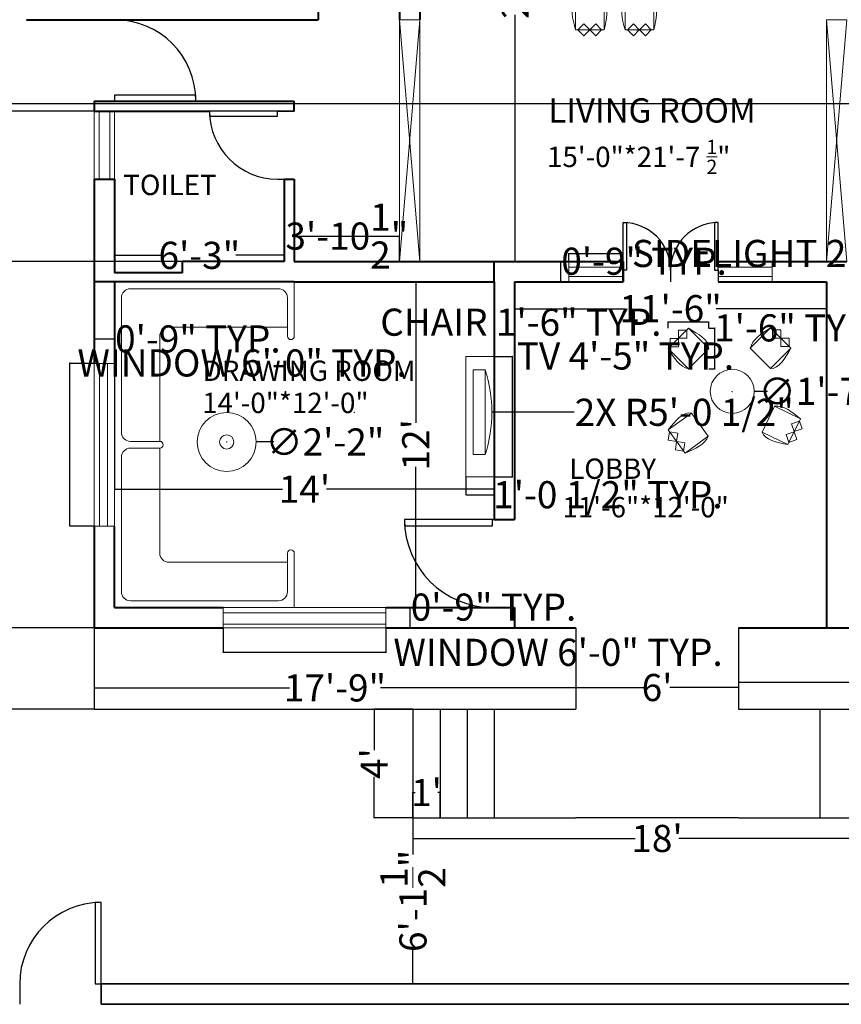
# Model space of a CAD drawing. Units: inches. Extents: x 1146 to 2917, y 889 to 2437.
# Tile 4 of 13: x 1428 to 1792, y 1432 to 1867. Entities that reach past the tile are written whole.
import ezdxf

# ---------------------------------------------------------------- set-up
doc = ezdxf.new("R2010")
doc.units = ezdxf.units.IN
doc.header["$MEASUREMENT"] = 0
for name, color, linetype, lineweight in [('A-ANNO-DIMS', 2, 'Continuous', 18), ('A-ANNO-SYMB', 7, 'Continuous', 25), ('A-AREA-IDEN', 7, 'Continuous', 18), ('A-FURN', 9, 'Continuous', 18), ('A-SITE-GATE', 10, 'Continuous', 25), ('A-SITE-WALL', 7, 'Continuous', 35), ('door', 10, 'Continuous', 25), ('openings', 130, 'Continuous', 18), ('staircase', 6, 'Continuous', 25), ('wall', 7, 'Continuous', 40), ('window', 5, 'Continuous', 18)]:
    doc.layers.add(name, color=color, linetype=linetype, lineweight=lineweight)
doc.styles.get("Standard").update_dxf_attribs({"font": 'arial.ttf'})
doc.dimstyles.get("Standard").update_dxf_attribs({"dimtxt": 12, "dimasz": 0.18, "dimexe": 0.18, "dimexo": 0.0625, "dimgap": 0.09, "dimtad": 0, "dimtoh": 1, "dimdec": 1, "dimzin": 0, "dimdsep": 46, "dimlunit": 4, "dimtxsty": 'Standard', "dimcen": 0.09, "dimadec": 0, "dimazin": 0, "dimtfac": 1, "dimtdec": 1, "dimtofl": 0, "dimtmove": 0, "dimatfit": 3, "dimfxl": 1, "dimtolj": 1, "dimtzin": 0, "dimarcsym": 0})

# ---------------------------------------------------------------- blocks, each defined once
blk = doc.blocks.new('*D9')
at = {"layer": 'A-ANNO-DIMS', "color": 0, "lineweight": -2, "transparency": 16777216}
for p, q in [((1674.13, 1598.33), (1674.13, 1571.83)), ((1746.13, 1598.33), (1746.13, 1571.83)), ((1674.31, 1572.01), (1704.49, 1572.01)), ((1745.95, 1572.01), (1715.78, 1572.01))]:
    blk.add_line(p, q, dxfattribs=at)
at = {"layer": 'A-ANNO-DIMS', "color": 0, "transparency": 16777216}
for points in [[(1674.31, 1572.04), (1674.31, 1571.98), (1674.13, 1572.01)], [(1745.95, 1572.04), (1745.95, 1571.98), (1746.13, 1572.01)]]:
    blk.add_solid(points, dxfattribs=at)
at = {"layer": 'Defpoints', "color": 0, "transparency": 16777216}
for p in [(1674.13, 1598.39), (1746.13, 1598.39), (1746.13, 1572.01)]:
    blk.add_point(p, dxfattribs=at)
at = {"layer": 'A-ANNO-DIMS', "color": 0, "transparency": 16777216, "insert": (1710.13, 1572.01), "char_height": 12, "attachment_point": 5}
blk.add_mtext("\\A1;6'", dxfattribs=at)
blk = doc.blocks.new('*D10')
at = {"layer": 'A-ANNO-DIMS', "color": 0, "lineweight": -2, "transparency": 16777216}
for p, q in [((1461.13, 1598.33), (1461.13, 1571.65)), ((1674.13, 1598.33), (1674.13, 1571.65)), ((1461.31, 1571.83), (1547.5, 1571.83)), ((1673.95, 1571.83), (1587.77, 1571.83))]:
    blk.add_line(p, q, dxfattribs=at)
at = {"layer": 'A-ANNO-DIMS', "color": 0, "transparency": 16777216}
for points in [[(1461.31, 1571.86), (1461.31, 1571.8), (1461.13, 1571.83)], [(1673.95, 1571.86), (1673.95, 1571.8), (1674.13, 1571.83)]]:
    blk.add_solid(points, dxfattribs=at)
at = {"layer": 'Defpoints', "color": 0, "transparency": 16777216}
for p in [(1461.13, 1598.39), (1674.13, 1598.39), (1674.13, 1571.83)]:
    blk.add_point(p, dxfattribs=at)
at = {"layer": 'A-ANNO-DIMS', "color": 0, "transparency": 16777216, "insert": (1567.63, 1571.83), "char_height": 12, "attachment_point": 5}
blk.add_mtext('\\A1;17\'-9"', dxfattribs=at)
blk = doc.blocks.new('*D11')
at = {"layer": 'A-ANNO-DIMS', "color": 0, "lineweight": -2, "transparency": 16777216}
for p, q in [((1746.13, 1598.33), (1746.13, 1574.21)), ((1959.13, 1598.33), (1959.13, 1574.21)), ((1746.31, 1574.39), (1832.5, 1574.39)), ((1958.95, 1574.39), (1872.77, 1574.39))]:
    blk.add_line(p, q, dxfattribs=at)
at = {"layer": 'A-ANNO-DIMS', "color": 0, "transparency": 16777216}
for points in [[(1746.31, 1574.42), (1746.31, 1574.36), (1746.13, 1574.39)], [(1958.95, 1574.42), (1958.95, 1574.36), (1959.13, 1574.39)]]:
    blk.add_solid(points, dxfattribs=at)
at = {"layer": 'Defpoints', "color": 0, "transparency": 16777216}
for p in [(1746.13, 1598.39), (1959.13, 1598.39), (1959.13, 1574.39)]:
    blk.add_point(p, dxfattribs=at)
at = {"layer": 'A-ANNO-DIMS', "color": 0, "transparency": 16777216, "insert": (1852.63, 1574.39), "char_height": 12, "attachment_point": 5}
blk.add_mtext('\\A1;17\'-9"', dxfattribs=at)
blk = doc.blocks.new('*D12')
at = {"layer": 'A-ANNO-DIMS', "color": 0, "lineweight": -2, "transparency": 16777216}
for p, q in [((1602.07, 1562.39), (1584.75, 1562.39)), ((1584.93, 1562.21), (1584.93, 1544.24)), ((1584.93, 1514.57), (1584.93, 1532.54)), ((1602.07, 1514.39), (1584.75, 1514.39))]:
    blk.add_line(p, q, dxfattribs=at)
at = {"layer": 'A-ANNO-DIMS', "color": 0, "transparency": 16777216}
for points in [[(1584.9, 1562.21), (1584.96, 1562.21), (1584.93, 1562.39)], [(1584.9, 1514.57), (1584.96, 1514.57), (1584.93, 1514.39)]]:
    blk.add_solid(points, dxfattribs=at)
at = {"layer": 'Defpoints', "color": 0, "transparency": 16777216}
for p in [(1602.13, 1562.39), (1584.93, 1514.39), (1602.13, 1514.39)]:
    blk.add_point(p, dxfattribs=at)
at = {"layer": 'A-ANNO-DIMS', "color": 0, "transparency": 16777216, "insert": (1584.93, 1538.39), "char_height": 12, "attachment_point": 5, "rotation": 90}
blk.add_mtext("\\A1;4'", dxfattribs=at)
blk = doc.blocks.new('*D13')
at = {"layer": 'A-ANNO-DIMS', "color": 0, "lineweight": -2, "transparency": 16777216}
for p, q in [((1602.13, 1514.45), (1602.13, 1525.77)), ((1602.31, 1525.59), (1603.09, 1525.59)), ((1613.95, 1525.59), (1613.18, 1525.59)), ((1614.13, 1514.45), (1614.13, 1525.77))]:
    blk.add_line(p, q, dxfattribs=at)
at = {"layer": 'A-ANNO-DIMS', "color": 0, "transparency": 16777216}
for points in [[(1602.31, 1525.62), (1602.31, 1525.56), (1602.13, 1525.59)], [(1613.95, 1525.62), (1613.95, 1525.56), (1614.13, 1525.59)]]:
    blk.add_solid(points, dxfattribs=at)
at = {"layer": 'Defpoints', "color": 0, "transparency": 16777216}
for p in [(1614.13, 1525.59), (1602.13, 1514.39), (1614.13, 1514.39)]:
    blk.add_point(p, dxfattribs=at)
at = {"layer": 'A-ANNO-DIMS', "color": 0, "transparency": 16777216, "insert": (1608.13, 1525.59), "char_height": 12, "attachment_point": 5}
blk.add_mtext("\\A1;1'", dxfattribs=at)
blk = doc.blocks.new('*D14')
at = {"layer": 'A-ANNO-DIMS', "color": 0, "lineweight": -2, "transparency": 16777216}
for p, q in [((1602.13, 1514.33), (1602.13, 1505.08)), ((1818.13, 1514.33), (1818.13, 1505.08)), ((1602.31, 1505.26), (1700.43, 1505.26)), ((1817.95, 1505.26), (1719.84, 1505.26))]:
    blk.add_line(p, q, dxfattribs=at)
at = {"layer": 'A-ANNO-DIMS', "color": 0, "transparency": 16777216}
for points in [[(1602.31, 1505.29), (1602.31, 1505.23), (1602.13, 1505.26)], [(1817.95, 1505.29), (1817.95, 1505.23), (1818.13, 1505.26)]]:
    blk.add_solid(points, dxfattribs=at)
at = {"layer": 'Defpoints', "color": 0, "transparency": 16777216}
for p in [(1602.13, 1514.39), (1818.13, 1514.39), (1818.13, 1505.26)]:
    blk.add_point(p, dxfattribs=at)
at = {"layer": 'A-ANNO-DIMS', "color": 0, "transparency": 16777216, "insert": (1710.13, 1505.26), "char_height": 12, "attachment_point": 5}
blk.add_mtext("\\A1;18'", dxfattribs=at)
blk = doc.blocks.new('*D15')
at = {"layer": 'A-ANNO-DIMS', "color": 0, "lineweight": -2, "transparency": 16777216}
for p, q in [((1602.07, 1514.39), (1601.95, 1514.39)), ((1602.13, 1514.21), (1602.13, 1498.09)), ((1602.13, 1441.07), (1602.13, 1457.19)), ((1602.07, 1440.89), (1601.95, 1440.89))]:
    blk.add_line(p, q, dxfattribs=at)
at = {"layer": 'A-ANNO-DIMS', "color": 0, "transparency": 16777216}
for points in [[(1602.1, 1514.21), (1602.16, 1514.21), (1602.13, 1514.39)], [(1602.1, 1441.07), (1602.16, 1441.07), (1602.13, 1440.89)]]:
    blk.add_solid(points, dxfattribs=at)
at = {"layer": 'Defpoints', "color": 0, "transparency": 16777216}
for p in [(1602.13, 1514.39), (1602.13, 1440.89), (1602.13, 1440.89)]:
    blk.add_point(p, dxfattribs=at)
at = {"layer": 'A-ANNO-DIMS', "color": 0, "transparency": 16777216, "insert": (1602.13, 1477.64), "char_height": 12, "attachment_point": 5, "rotation": 90}
blk.add_mtext('\\A1;6\'-1{\\H1x;\\S1/2;}"', dxfattribs=at)
blk = doc.blocks.new('*U22')
for p, q in [((-24, 0), (-24, -6)), ((0, 0), (0, -6))]:
    blk.add_line(p, q)
blk.add_lwpolyline([(0, 0), (0, 24), (-1.75, 24), (-1.75, 0)], close=True)
blk.add_arc((0, 0), 24, 90, 180)
blk = doc.blocks.new('*U18')
for p, q in [((-24, 0), (-24, -6)), ((0, 0), (0, -6))]:
    blk.add_line(p, q)
blk.add_lwpolyline([(0, 0), (0, 24), (-1.75, 24), (-1.75, 0)], close=True)
blk.add_arc((0, 0), 24, 90, 180)
blk = doc.blocks.new('*U21')
for p, q in [((0, 0), (0, 6)), ((24, 0), (24, 6))]:
    blk.add_line(p, q)
blk.add_lwpolyline([(0, 0), (0, -24), (1.75, -24), (1.75, 0)], close=True)
blk.add_arc((0, 0), 24, 270, 0)
blk = doc.blocks.new('*D32')
at = {"layer": 'A-ANNO-DIMS', "color": 0, "lineweight": -2, "transparency": 16777216}
for p, q in [((1470.13, 1760.45), (1470.13, 1763.35)), ((1470.31, 1763.17), (1491.56, 1763.17)), ((1544.95, 1763.17), (1523.71, 1763.17)), ((1545.13, 1760.45), (1545.13, 1763.35))]:
    blk.add_line(p, q, dxfattribs=at)
at = {"layer": 'A-ANNO-DIMS', "color": 0, "transparency": 16777216}
for points in [[(1470.31, 1763.2), (1470.31, 1763.14), (1470.13, 1763.17)], [(1544.95, 1763.2), (1544.95, 1763.14), (1545.13, 1763.17)]]:
    blk.add_solid(points, dxfattribs=at)
at = {"layer": 'Defpoints', "color": 0, "transparency": 16777216}
for p in [(1470.13, 1763.17), (1470.13, 1760.39), (1545.13, 1760.39)]:
    blk.add_point(p, dxfattribs=at)
at = {"layer": 'A-ANNO-DIMS', "color": 0, "transparency": 16777216, "insert": (1507.63, 1763.17), "char_height": 12, "attachment_point": 5}
blk.add_mtext('\\A1;6\'-3"', dxfattribs=at)
blk = doc.blocks.new('*D33')
at = {"layer": 'A-ANNO-DIMS', "color": 0, "lineweight": -2, "transparency": 16777216}
for p, q in [((1549.63, 1760.45), (1549.63, 1771.86)), ((1549.81, 1771.68), (1595.95, 1771.68)), ((1596.13, 1760.45), (1596.13, 1771.86))]:
    blk.add_line(p, q, dxfattribs=at)
at = {"layer": 'A-ANNO-DIMS', "color": 0, "transparency": 16777216}
for points in [[(1549.81, 1771.71), (1549.81, 1771.65), (1549.63, 1771.68)], [(1595.95, 1771.71), (1595.95, 1771.65), (1596.13, 1771.68)]]:
    blk.add_solid(points, dxfattribs=at)
at = {"layer": 'Defpoints', "color": 0, "transparency": 16777216}
for p in [(1596.13, 1771.68), (1549.63, 1760.39), (1596.13, 1760.39)]:
    blk.add_point(p, dxfattribs=at)
at = {"layer": 'A-ANNO-DIMS', "color": 0, "transparency": 16777216, "insert": (1572.88, 1771.68), "char_height": 12, "attachment_point": 5}
blk.add_mtext('\\A1;3\'-10{\\H1x;\\S1/2;}"', dxfattribs=at)
blk = doc.blocks.new('*D39')
at = {"layer": 'A-ANNO-DIMS', "color": 0, "lineweight": -2, "transparency": 16777216}
for p, q in [((1605.2, 2020.39), (1647.47, 2020.39)), ((1647.29, 2020.21), (1647.29, 1911.2)), ((1647.29, 1760.57), (1647.29, 1869.59)), ((1605.2, 1760.39), (1647.47, 1760.39))]:
    blk.add_line(p, q, dxfattribs=at)
at = {"layer": 'A-ANNO-DIMS', "color": 0, "transparency": 16777216}
for points in [[(1647.26, 2020.21), (1647.32, 2020.21), (1647.29, 2020.39)], [(1647.26, 1760.57), (1647.32, 1760.57), (1647.29, 1760.39)]]:
    blk.add_solid(points, dxfattribs=at)
at = {"layer": 'Defpoints', "color": 0, "transparency": 16777216}
for p in [(1605.13, 2020.39), (1605.13, 1760.39), (1647.29, 1760.39)]:
    blk.add_point(p, dxfattribs=at)
at = {"layer": 'A-ANNO-DIMS', "color": 0, "transparency": 16777216, "insert": (1647.29, 1890.39), "char_height": 12, "attachment_point": 5, "rotation": 90}
blk.add_mtext('\\A1;21\'-8"', dxfattribs=at)
blk = doc.blocks.new('*D40')
at = {"layer": 'A-ANNO-DIMS', "color": 0, "lineweight": -2, "transparency": 16777216}
for p, q in [((1470.13, 1751.33), (1470.13, 1659.58)), ((1638.13, 1751.33), (1638.13, 1659.58)), ((1470.31, 1659.76), (1544.43, 1659.76)), ((1637.95, 1659.76), (1563.84, 1659.76))]:
    blk.add_line(p, q, dxfattribs=at)
at = {"layer": 'A-ANNO-DIMS', "color": 0, "transparency": 16777216}
for points in [[(1470.31, 1659.79), (1470.31, 1659.73), (1470.13, 1659.76)], [(1637.95, 1659.79), (1637.95, 1659.73), (1638.13, 1659.76)]]:
    blk.add_solid(points, dxfattribs=at)
at = {"layer": 'Defpoints', "color": 0, "transparency": 16777216}
for p in [(1470.13, 1751.39), (1638.13, 1751.39), (1638.13, 1659.76)]:
    blk.add_point(p, dxfattribs=at)
at = {"layer": 'A-ANNO-DIMS', "color": 0, "transparency": 16777216, "insert": (1554.13, 1659.76), "char_height": 12, "attachment_point": 5}
blk.add_mtext("\\A1;14'", dxfattribs=at)
blk = doc.blocks.new('*D41')
at = {"layer": 'A-ANNO-DIMS', "color": 0, "lineweight": -2, "transparency": 16777216}
for p, q in [((1638.07, 1751.39), (1603.2, 1751.39)), ((1603.38, 1751.21), (1603.38, 1689.1)), ((1603.38, 1607.57), (1603.38, 1669.68)), ((1638.07, 1607.39), (1603.2, 1607.39))]:
    blk.add_line(p, q, dxfattribs=at)
at = {"layer": 'A-ANNO-DIMS', "color": 0, "transparency": 16777216}
for points in [[(1603.35, 1751.21), (1603.41, 1751.21), (1603.38, 1751.39)], [(1603.35, 1607.57), (1603.41, 1607.57), (1603.38, 1607.39)]]:
    blk.add_solid(points, dxfattribs=at)
at = {"layer": 'Defpoints', "color": 0, "transparency": 16777216}
for p in [(1638.13, 1751.39), (1603.38, 1607.39), (1638.13, 1607.39)]:
    blk.add_point(p, dxfattribs=at)
at = {"layer": 'A-ANNO-DIMS', "color": 0, "transparency": 16777216, "insert": (1603.38, 1679.39), "char_height": 12, "attachment_point": 5, "rotation": 90}
blk.add_mtext("\\A1;12'", dxfattribs=at)
blk = doc.blocks.new('*D44')
at = {"layer": 'A-ANNO-DIMS', "color": 0, "lineweight": -2, "transparency": 16777216}
for p, q in [((1647.13, 1751.33), (1647.13, 1739.39)), ((1785.13, 1751.33), (1785.13, 1739.39)), ((1647.31, 1739.57), (1696, 1739.57)), ((1784.95, 1739.57), (1736.27, 1739.57))]:
    blk.add_line(p, q, dxfattribs=at)
at = {"layer": 'A-ANNO-DIMS', "color": 0, "transparency": 16777216}
for points in [[(1647.31, 1739.6), (1647.31, 1739.54), (1647.13, 1739.57)], [(1784.95, 1739.6), (1784.95, 1739.54), (1785.13, 1739.57)]]:
    blk.add_solid(points, dxfattribs=at)
at = {"layer": 'Defpoints', "color": 0, "transparency": 16777216}
for p in [(1647.13, 1751.39), (1785.13, 1751.39), (1785.13, 1739.57)]:
    blk.add_point(p, dxfattribs=at)
at = {"layer": 'A-ANNO-DIMS', "color": 0, "transparency": 16777216, "insert": (1716.13, 1739.57), "char_height": 12, "attachment_point": 5}
blk.add_mtext('\\A1;11\'-6"', dxfattribs=at)
blk = doc.blocks.new('*U17')
for p, q in [((0, 0), (0, -6)), ((24, 0), (24, -6))]:
    blk.add_line(p, q)
blk.add_lwpolyline([(0, 0), (0, 24), (1.75, 24), (1.75, 0)], close=True)
blk.add_arc((0, 0), 24, 0, 90)
blk = doc.blocks.new('CHAIR-LOUNGE')
blk.add_line((0, 8.98), (8.98, 0))
blk.add_lwpolyline([(0, 8.98), (8.98, 17.96), (17.96, 8.98), (8.98, 0)])
for points in [[(9.79, 17.15), (13.47, 17.15), (13.47, 13.47), (9.79, 13.47)], [(13.52, 13.42), (17.2, 13.42), (17.2, 9.74), (13.52, 9.74)]]:
    blk.add_lwpolyline(points, close=True)
for points in [[(8.98, 17.96), (4.93, 15.41), (0.87, 12.85), (0, 8.98)], [(17.96, 8.98), (15.38, 4.49), (12.8, -0.01), (8.98, 0)]]:
    blk.add_open_spline(points, degree=3)
blk = doc.blocks.new('TV-CONSOLE')
for points in [[(0, 53.2), (12.54, 53.2), (12.54, 0), (0, 0)], [(3.13, 47.21), (8.47, 47.21), (8.47, 9.76), (3.13, 9.76)]]:
    blk.add_lwpolyline(points, close=True)
blk.add_arc((-49.25, 28.49), 60.68, 342.0216, 17.9784)
blk = doc.blocks.new('WINDOW-PLAN-72-3')
for points in [[(0, 72), (9, 72), (9, 0), (0, 0)], [(2.34, 72), (5.93, 72), (5.93, 0), (2.34, 0)]]:
    blk.add_lwpolyline(points, close=True)
blk = doc.blocks.new('WINDOW-PLAN-72-4')
for points in [[(0, 9), (72, 9), (72, 0), (0, 0)], [(0, 6.62), (72, 6.62), (72, 1.59), (0, 1.59)]]:
    blk.add_lwpolyline(points, close=True)
blk = doc.blocks.new('SIDELIGHT-PLAN-24')
for points in [[(0, 9), (24, 9), (24, 0), (0, 0)], [(0, 6.5), (24, 6.5), (24, 2.47), (0, 2.47)]]:
    blk.add_lwpolyline(points, close=True)
blk = doc.blocks.new('*D97')
at = {"layer": 'A-ANNO-DIMS', "color": 0, "lineweight": -2, "transparency": 16777216}
for p, q in [((1715.06, 1733.6), (1714.88, 1733.6)), ((1715.06, 1730.96), (1715.06, 1733.78)), ((1732.85, 1733.6), (1715.24, 1733.6)), ((1733.03, 1730.96), (1733.03, 1733.78))]:
    blk.add_line(p, q, dxfattribs=at)
at = {"layer": 'A-ANNO-DIMS', "color": 0, "transparency": 16777216}
for points in [[(1715.24, 1733.63), (1715.24, 1733.57), (1715.06, 1733.6)], [(1732.85, 1733.63), (1732.85, 1733.57), (1733.03, 1733.6)]]:
    blk.add_solid(points, dxfattribs=at)
at = {"layer": 'Defpoints', "color": 0, "transparency": 16777216}
for p in [(1715.06, 1733.6), (1715.06, 1730.9), (1733.03, 1730.9)]:
    blk.add_point(p, dxfattribs=at)
at = {"layer": 'A-ANNO-DIMS', "color": 0, "transparency": 16777216, "insert": (1649.87, 1733.6), "char_height": 12, "attachment_point": 5}
blk.add_mtext('\\A1;CHAIR 1\'-6" TYP.', dxfattribs=at)
blk = doc.blocks.new('*D98')
at = {"layer": 'A-ANNO-DIMS', "color": 0, "lineweight": -2, "transparency": 16777216}
for p, q in [((1733.09, 1730.9), (1735.9, 1730.9)), ((1735.72, 1730.9), (1735.72, 1731.08)), ((1735.72, 1731.08), (1735.9, 1731.08)), ((1735.72, 1713.12), (1735.72, 1730.72)), ((1733.09, 1712.94), (1735.9, 1712.94))]:
    blk.add_line(p, q, dxfattribs=at)
at = {"layer": 'A-ANNO-DIMS', "color": 0, "transparency": 16777216}
for points in [[(1735.69, 1730.72), (1735.75, 1730.72), (1735.72, 1730.9)], [(1735.69, 1713.12), (1735.75, 1713.12), (1735.72, 1712.94)]]:
    blk.add_solid(points, dxfattribs=at)
at = {"layer": 'Defpoints', "color": 0, "transparency": 16777216}
for p in [(1733.03, 1730.9), (1735.72, 1730.9), (1733.03, 1712.94)]:
    blk.add_point(p, dxfattribs=at)
at = {"layer": 'A-ANNO-DIMS', "color": 0, "transparency": 16777216, "insert": (1772, 1731.08), "char_height": 12, "attachment_point": 5}
blk.add_mtext('\\A1;1\'-6" TYP.', dxfattribs=at)
blk = doc.blocks.new('*D107')
at = {"layer": 'A-ANNO-DIMS', "color": 0, "lineweight": -2, "transparency": 16777216}
for p, q in [((1638.2, 1718.46), (1646.29, 1718.46)), ((1646.11, 1718.46), (1646.11, 1718.64)), ((1646.11, 1718.64), (1646.29, 1718.64)), ((1646.11, 1665.44), (1646.11, 1718.28)), ((1638.2, 1665.26), (1646.29, 1665.26))]:
    blk.add_line(p, q, dxfattribs=at)
at = {"layer": 'A-ANNO-DIMS', "color": 0, "transparency": 16777216}
for points in [[(1646.08, 1718.28), (1646.14, 1718.28), (1646.11, 1718.46)], [(1646.08, 1665.44), (1646.14, 1665.44), (1646.11, 1665.26)]]:
    blk.add_solid(points, dxfattribs=at)
at = {"layer": 'Defpoints', "color": 0, "transparency": 16777216}
for p in [(1638.13, 1718.46), (1646.11, 1718.46), (1638.13, 1665.26)]:
    blk.add_point(p, dxfattribs=at)
at = {"layer": 'A-ANNO-DIMS', "color": 0, "transparency": 16777216, "insert": (1696.15, 1718.64), "char_height": 12, "attachment_point": 5}
blk.add_mtext('\\A1;TV 4\'-5" TYP.', dxfattribs=at)
blk = doc.blocks.new('*D108')
at = {"layer": 'A-ANNO-DIMS', "color": 0, "lineweight": -2, "transparency": 16777216}
for p, q in [((1625.59, 1665.19), (1625.59, 1657.1)), ((1638.13, 1665.19), (1638.13, 1657.1)), ((1625.77, 1657.28), (1637.95, 1657.28)), ((1638.13, 1657.28), (1638.31, 1657.28))]:
    blk.add_line(p, q, dxfattribs=at)
at = {"layer": 'A-ANNO-DIMS', "color": 0, "transparency": 16777216}
for points in [[(1625.77, 1657.31), (1625.77, 1657.25), (1625.59, 1657.28)], [(1637.95, 1657.31), (1637.95, 1657.25), (1638.13, 1657.28)]]:
    blk.add_solid(points, dxfattribs=at)
at = {"layer": 'Defpoints', "color": 0, "transparency": 16777216}
for p in [(1625.59, 1665.26), (1638.13, 1665.26), (1638.13, 1657.28)]:
    blk.add_point(p, dxfattribs=at)
at = {"layer": 'A-ANNO-DIMS', "color": 0, "transparency": 16777216, "insert": (1688.39, 1657.28), "char_height": 12, "attachment_point": 5}
blk.add_mtext('\\A1;1\'-0 1/2" TYP.', dxfattribs=at)
blk = doc.blocks.new('*D113')
at = {"layer": 'A-ANNO-DIMS', "color": 0, "lineweight": -2, "transparency": 16777216}
for p, q in [((1461.07, 1715.39), (1450.15, 1715.39)), ((1450.33, 1715.39), (1450.33, 1715.57)), ((1450.33, 1715.57), (1450.51, 1715.57)), ((1450.33, 1643.57), (1450.33, 1715.21)), ((1461.07, 1643.39), (1450.15, 1643.39))]:
    blk.add_line(p, q, dxfattribs=at)
at = {"layer": 'A-ANNO-DIMS', "color": 0, "transparency": 16777216}
for points in [[(1450.3, 1715.21), (1450.36, 1715.21), (1450.33, 1715.39)], [(1450.3, 1643.57), (1450.36, 1643.57), (1450.33, 1643.39)]]:
    blk.add_solid(points, dxfattribs=at)
at = {"layer": 'Defpoints', "color": 0, "transparency": 16777216}
for p in [(1450.33, 1715.39), (1461.13, 1715.39), (1461.13, 1643.39)]:
    blk.add_point(p, dxfattribs=at)
at = {"layer": 'A-ANNO-DIMS', "color": 0, "transparency": 16777216, "insert": (1526.53, 1715.57), "char_height": 12, "attachment_point": 5}
blk.add_mtext('\\A1;WINDOW 6\'-0" TYP.', dxfattribs=at)
blk = doc.blocks.new('*D114')
at = {"layer": 'A-ANNO-DIMS', "color": 0, "lineweight": -2, "transparency": 16777216}
for p, q in [((1461.13, 1715.45), (1461.13, 1726.37)), ((1461.31, 1726.19), (1469.95, 1726.19)), ((1470.13, 1715.45), (1470.13, 1726.37)), ((1470.13, 1726.19), (1470.31, 1726.19))]:
    blk.add_line(p, q, dxfattribs=at)
at = {"layer": 'A-ANNO-DIMS', "color": 0, "transparency": 16777216}
for points in [[(1461.31, 1726.22), (1461.31, 1726.16), (1461.13, 1726.19)], [(1469.95, 1726.22), (1469.95, 1726.16), (1470.13, 1726.19)]]:
    blk.add_solid(points, dxfattribs=at)
at = {"layer": 'Defpoints', "color": 0, "transparency": 16777216}
for p in [(1470.13, 1726.19), (1461.13, 1715.39), (1470.13, 1715.39)]:
    blk.add_point(p, dxfattribs=at)
at = {"layer": 'A-ANNO-DIMS', "color": 0, "transparency": 16777216, "insert": (1506.98, 1726.19), "char_height": 12, "attachment_point": 5}
blk.add_mtext('\\A1;0\'-9" TYP.', dxfattribs=at)
blk = doc.blocks.new('*D115')
at = {"layer": 'A-ANNO-DIMS', "color": 0, "lineweight": -2, "transparency": 16777216}
for p, q in [((1518.13, 1598.33), (1518.13, 1587.41)), ((1590.13, 1598.33), (1590.13, 1587.41)), ((1518.31, 1587.59), (1589.95, 1587.59)), ((1590.13, 1587.59), (1590.31, 1587.59))]:
    blk.add_line(p, q, dxfattribs=at)
at = {"layer": 'A-ANNO-DIMS', "color": 0, "transparency": 16777216}
for points in [[(1518.31, 1587.62), (1518.31, 1587.56), (1518.13, 1587.59)], [(1589.95, 1587.62), (1589.95, 1587.56), (1590.13, 1587.59)]]:
    blk.add_solid(points, dxfattribs=at)
at = {"layer": 'Defpoints', "color": 0, "transparency": 16777216}
for p in [(1518.13, 1598.39), (1590.13, 1598.39), (1590.13, 1587.59)]:
    blk.add_point(p, dxfattribs=at)
at = {"layer": 'A-ANNO-DIMS', "color": 0, "transparency": 16777216, "insert": (1666.33, 1587.59), "char_height": 12, "attachment_point": 5}
blk.add_mtext('\\A1;WINDOW 6\'-0" TYP.', dxfattribs=at)
blk = doc.blocks.new('*D116')
at = {"layer": 'A-ANNO-DIMS', "color": 0, "lineweight": -2, "transparency": 16777216}
for p, q in [((1590.2, 1607.39), (1601.11, 1607.39)), ((1600.93, 1607.39), (1600.93, 1607.57)), ((1600.93, 1607.57), (1601.11, 1607.57)), ((1600.93, 1598.57), (1600.93, 1607.21)), ((1590.2, 1598.39), (1601.11, 1598.39))]:
    blk.add_line(p, q, dxfattribs=at)
at = {"layer": 'A-ANNO-DIMS', "color": 0, "transparency": 16777216}
for points in [[(1600.9, 1607.21), (1600.96, 1607.21), (1600.93, 1607.39)], [(1600.9, 1598.57), (1600.96, 1598.57), (1600.93, 1598.39)]]:
    blk.add_solid(points, dxfattribs=at)
at = {"layer": 'Defpoints', "color": 0, "transparency": 16777216}
for p in [(1590.13, 1607.39), (1600.93, 1607.39), (1590.13, 1598.39)]:
    blk.add_point(p, dxfattribs=at)
at = {"layer": 'A-ANNO-DIMS', "color": 0, "transparency": 16777216, "insert": (1637.78, 1607.57), "char_height": 12, "attachment_point": 5}
blk.add_mtext('\\A1;0\'-9" TYP.', dxfattribs=at)
blk = doc.blocks.new('*D117')
at = {"layer": 'A-ANNO-DIMS', "color": 0, "lineweight": -2, "transparency": 16777216}
for p, q in [((1671.13, 1760.45), (1671.13, 1764.17)), ((1671.31, 1763.99), (1694.95, 1763.99)), ((1695.13, 1760.45), (1695.13, 1764.17)), ((1695.13, 1763.99), (1695.31, 1763.99))]:
    blk.add_line(p, q, dxfattribs=at)
at = {"layer": 'A-ANNO-DIMS', "color": 0, "transparency": 16777216}
for points in [[(1671.31, 1764.02), (1671.31, 1763.96), (1671.13, 1763.99)], [(1694.95, 1764.02), (1694.95, 1763.96), (1695.13, 1763.99)]]:
    blk.add_solid(points, dxfattribs=at)
at = {"layer": 'Defpoints', "color": 0, "transparency": 16777216}
for p in [(1695.13, 1763.99), (1671.13, 1760.39), (1695.13, 1760.39)]:
    blk.add_point(p, dxfattribs=at)
at = {"layer": 'A-ANNO-DIMS', "color": 0, "transparency": 16777216, "insert": (1778.52, 1763.99), "char_height": 12, "attachment_point": 5}
blk.add_mtext('\\A1;SIDELIGHT 2\'-0" TYP.', dxfattribs=at)
blk = doc.blocks.new('*D118')
at = {"layer": 'A-ANNO-DIMS', "color": 0, "lineweight": -2, "transparency": 16777216}
for p, q in [((1671.07, 1760.39), (1667.35, 1760.39)), ((1667.53, 1760.39), (1667.53, 1760.57)), ((1667.53, 1760.57), (1667.71, 1760.57)), ((1667.53, 1751.57), (1667.53, 1760.21)), ((1671.07, 1751.39), (1667.35, 1751.39))]:
    blk.add_line(p, q, dxfattribs=at)
at = {"layer": 'A-ANNO-DIMS', "color": 0, "transparency": 16777216}
for points in [[(1667.5, 1760.21), (1667.56, 1760.21), (1667.53, 1760.39)], [(1667.5, 1751.57), (1667.56, 1751.57), (1667.53, 1751.39)]]:
    blk.add_solid(points, dxfattribs=at)
at = {"layer": 'Defpoints', "color": 0, "transparency": 16777216}
for p in [(1667.53, 1760.39), (1671.13, 1760.39), (1671.13, 1751.39)]:
    blk.add_point(p, dxfattribs=at)
at = {"layer": 'A-ANNO-DIMS', "color": 0, "transparency": 16777216, "insert": (1704.38, 1760.57), "char_height": 12, "attachment_point": 5}
blk.add_mtext('\\A1;0\'-9" TYP.', dxfattribs=at)
blk = doc.blocks.new('*D170')
at = {"layer": 'A-ANNO-DIMS', "color": 0, "lineweight": -2, "transparency": 16777216}
for p, q in [((1461.07, 1598.39), (1163.51, 1598.39)), ((1163.69, 1598.21), (1163.69, 1596.43)), ((1163.69, 1562.57), (1163.69, 1564.36)), ((1461.07, 1562.39), (1163.51, 1562.39))]:
    blk.add_line(p, q, dxfattribs=at)
at = {"layer": 'A-ANNO-DIMS', "color": 0, "transparency": 16777216}
for points in [[(1163.66, 1598.21), (1163.72, 1598.21), (1163.69, 1598.39)], [(1163.66, 1562.57), (1163.72, 1562.57), (1163.69, 1562.39)]]:
    blk.add_solid(points, dxfattribs=at)
at = {"layer": 'Defpoints', "color": 0, "transparency": 16777216}
for p in [(1461.13, 1598.39), (1163.69, 1562.39), (1461.13, 1562.39)]:
    blk.add_point(p, dxfattribs=at)
at = {"layer": 'A-ANNO-DIMS', "color": 0, "transparency": 16777216, "insert": (1163.69, 1580.39), "char_height": 12, "attachment_point": 5, "rotation": 90}
blk.add_mtext('\\A1;3\'-0"', dxfattribs=at)
blk = doc.blocks.new('*D171')
at = {"layer": 'A-ANNO-DIMS', "color": 0, "lineweight": -2, "transparency": 16777216}
for p, q in [((1549.57, 1826.89), (1163.51, 1826.89)), ((1163.69, 1826.71), (1163.69, 1823.66)), ((1545.07, 1760.39), (1163.51, 1760.39)), ((1163.69, 1760.57), (1163.69, 1763.62))]:
    blk.add_line(p, q, dxfattribs=at)
at = {"layer": 'A-ANNO-DIMS', "color": 0, "transparency": 16777216}
for points in [[(1163.66, 1826.71), (1163.72, 1826.71), (1163.69, 1826.89)], [(1163.66, 1760.57), (1163.72, 1760.57), (1163.69, 1760.39)]]:
    blk.add_solid(points, dxfattribs=at)
at = {"layer": 'Defpoints', "color": 0, "transparency": 16777216}
for p in [(1549.63, 1826.89), (1163.69, 1760.39), (1545.13, 1760.39)]:
    blk.add_point(p, dxfattribs=at)
at = {"layer": 'A-ANNO-DIMS', "color": 0, "transparency": 16777216, "insert": (1163.69, 1793.64), "char_height": 12, "attachment_point": 5, "rotation": 90}
blk.add_mtext('\\A1;5\'-6 1/2"', dxfattribs=at)
blk = doc.blocks.new('*D176')
at = {"layer": 'A-ANNO-DIMS', "color": 0, "lineweight": -2, "transparency": 16777216}
for p, q in [((1576.25, 1693.74), (1576.43, 1693.74)), ((1576.34, 1693.65), (1576.34, 1693.83)), ((1673.42, 1693.74), (1637.2, 1693.74))]:
    blk.add_line(p, q, dxfattribs=at)
at = {"layer": 'A-ANNO-DIMS', "color": 0, "transparency": 16777216}
blk.add_solid([(1637.2, 1693.77), (1637.2, 1693.71), (1637.02, 1693.74)], dxfattribs=at)
at = {"layer": 'Defpoints', "color": 0, "transparency": 16777216}
for p in [(1576.34, 1693.74), (1637.02, 1693.74)]:
    blk.add_point(p, dxfattribs=at)
at = {"layer": 'A-ANNO-DIMS', "color": 0, "transparency": 16777216, "insert": (1722.18, 1693.74), "char_height": 12, "attachment_point": 5}
blk.add_mtext('\\A1;2X R5\'-0 1/2"', dxfattribs=at)
blk = doc.blocks.new('*D179')
at = {"layer": 'A-ANNO-DIMS', "color": 0, "lineweight": -2, "transparency": 16777216}
for p, q in [((1519.64, 1680.61), (1519.82, 1680.61)), ((1519.73, 1680.52), (1519.73, 1680.7)), ((1540.64, 1680.61), (1532.98, 1680.61))]:
    blk.add_line(p, q, dxfattribs=at)
at = {"layer": 'A-ANNO-DIMS', "color": 0, "transparency": 16777216}
blk.add_solid([(1532.98, 1680.64), (1532.98, 1680.58), (1532.8, 1680.61)], dxfattribs=at)
at = {"layer": 'Defpoints', "color": 0, "transparency": 16777216}
for p in [(1506.66, 1680.61), (1532.8, 1680.61)]:
    blk.add_point(p, dxfattribs=at)
at = {"layer": 'A-ANNO-DIMS', "color": 0, "transparency": 16777216, "insert": (1563.2, 1680.61), "char_height": 12, "attachment_point": 5}
blk.add_mtext('\\A1;∅2\'-2"', dxfattribs=at)
blk = doc.blocks.new('*D181')
at = {"layer": 'A-ANNO-DIMS', "color": 0, "lineweight": -2, "transparency": 16777216}
for p, q in [((1743.32, 1703), (1743.5, 1703)), ((1743.41, 1702.91), (1743.41, 1703.09)), ((1758.97, 1703), (1753.31, 1703))]:
    blk.add_line(p, q, dxfattribs=at)
at = {"layer": 'A-ANNO-DIMS', "color": 0, "transparency": 16777216}
blk.add_solid([(1753.31, 1703.03), (1753.31, 1702.97), (1753.13, 1703)], dxfattribs=at)
at = {"layer": 'Defpoints', "color": 0, "transparency": 16777216}
for p in [(1733.68, 1703), (1753.13, 1703)]:
    blk.add_point(p, dxfattribs=at)
at = {"layer": 'A-ANNO-DIMS', "color": 0, "transparency": 16777216, "insert": (1795.52, 1703), "char_height": 12, "attachment_point": 5}
blk.add_mtext('\\A1;∅1\'-7 1/2"', dxfattribs=at)

msp = doc.modelspace()

# ---------------------------------------------------------------- linework, layer by layer
at = {"layer": 'A-ANNO-SYMB'}
msp.add_line((1232.84, 1830.35), (2074.15, 1830.35), dxfattribs=at)
at = {"layer": 'A-FURN'}
for p, q in [((1549.63, 1751.39), (1549.63, 1727.39)), ((1542.63, 1748.39), (1477.13, 1748.39)), ((1473.13, 1744.39), (1473.13, 1684.89)), ((1546.63, 1744.39), (1546.63, 1727.39)), ((1546.63, 1731.39), (1494.13, 1731.39)), ((1490.13, 1727.39), (1490.13, 1680.89)), ((1477.13, 1680.89), (1490.13, 1680.89)), ((1477.13, 1677.89), (1490.13, 1677.89)), ((1490.13, 1677.89), (1490.13, 1631.39)), ((1473.13, 1673.89), (1473.13, 1614.39)), ((1546.63, 1614.39), (1546.63, 1631.39)), ((1549.63, 1607.39), (1549.63, 1631.39)), ((1494.13, 1627.39), (1546.63, 1627.39)), ((1477.13, 1610.39), (1542.63, 1610.39))]:
    msp.add_line(p, q, dxfattribs=at)
for centre, radius in [((1743.41, 1703), 9.73), ((1519.73, 1680.61), 13.07), ((1519.73, 1680.61), 3.13)]:
    msp.add_circle(centre, radius, dxfattribs=at)
for centre, radius, start, end in [((1477.13, 1744.39), 4, 90, 180), ((1542.63, 1744.39), 4, 0, 90), ((1494.13, 1727.39), 4, 90, 180), ((1548.13, 1727.39), 1.5, 180, 0), ((1477.13, 1684.89), 4, 180, 270), ((1477.13, 1673.89), 4, 90, 180), ((1490.13, 1679.39), 1.5, 270, 90), ((1494.13, 1631.39), 4, 180, 270), ((1548.13, 1631.39), 1.5, 0, 180), ((1477.13, 1614.39), 4, 180, 270), ((1542.63, 1614.39), 4, 270, 0)]:
    msp.add_arc(centre, radius, start, end, dxfattribs=at)
at = {"layer": 'A-SITE-WALL'}
for p, q in [((1464.13, 1440.89), (1464.13, 1431.89)), ((1464.13, 1440.89), (1896.13, 1440.89)), ((1464.13, 1431.89), (1896.13, 1431.89))]:
    msp.add_line(p, q, dxfattribs=at)
at = {"layer": 'openings'}
for p, q in [((1596.13, 1867.39), (1596.13, 1760.39)), ((1596.13, 1867.39), (1605.13, 1760.39)), ((1596.13, 1760.39), (1605.13, 1867.39)), ((1605.13, 1867.39), (1596.13, 1867.39)), ((1605.13, 1760.39), (1605.13, 1867.39)), ((1785.13, 1867.39), (1785.13, 1760.39)), ((1785.13, 1867.39), (1794.13, 1760.39)), ((1785.13, 1760.39), (1794.13, 1867.39)), ((1785.13, 1867.39), (1794.13, 1867.39)), ((1605.13, 1760.39), (1596.13, 1760.39)), ((1794.13, 1760.39), (1785.13, 1760.39))]:
    msp.add_line(p, q, dxfattribs=at)
at = {"layer": 'staircase'}
for p, q in [((1461.13, 1598.39), (1461.13, 1562.39)), ((1674.13, 1598.39), (1674.13, 1562.39)), ((1746.13, 1598.39), (1746.13, 1562.39)), ((1461.13, 1562.39), (1674.13, 1562.39)), ((1602.13, 1562.39), (1602.13, 1514.39)), ((1614.13, 1562.39), (1614.13, 1514.39)), ((1626.13, 1562.39), (1626.13, 1514.39)), ((1638.13, 1562.39), (1638.13, 1514.39)), ((1746.13, 1562.39), (1959.13, 1562.39)), ((1782.13, 1562.39), (1782.13, 1514.39)), ((1602.13, 1514.39), (1674.13, 1514.39)), ((1746.13, 1514.39), (1674.13, 1514.39)), ((1746.13, 1514.39), (1818.13, 1514.39))]:
    msp.add_line(p, q, dxfattribs=at)
at = {"layer": 'wall'}
for p, q in [((1596.13, 2020.39), (1596.13, 1867.39)), ((1605.13, 2020.39), (1605.13, 1867.39)), ((1560.13, 1876.39), (1560.13, 1867.39)), ((1431.13, 1867.39), (1560.13, 1867.39)), ((1461.13, 1831.39), (1461.13, 1826.89)), ((1461.13, 1831.39), (1549.63, 1831.39)), ((1549.63, 1826.89), (1549.63, 1831.39)), ((1461.13, 1826.89), (1512.13, 1826.89)), ((1461.13, 1796.89), (1470.13, 1796.89)), ((1461.13, 1796.89), (1461.13, 1715.39)), ((1470.13, 1796.89), (1470.13, 1755.39)), ((1545.13, 1796.89), (1545.13, 1760.39)), ((1545.13, 1796.89), (1549.63, 1796.89)), ((1549.63, 1796.89), (1549.63, 1760.39)), ((1545.13, 1760.39), (1500.12, 1760.39)), ((1500.12, 1755.39), (1500.12, 1760.39)), ((1549.63, 1760.39), (1695.13, 1760.39)), ((1638.13, 1751.39), (1638.13, 1760.39)), ((1695.13, 1751.39), (1695.13, 1760.39)), ((1695.13, 1760.39), (1695.13, 1751.39)), ((1737.13, 1760.39), (1794.13, 1760.39)), ((1500.12, 1755.39), (1470.13, 1755.39)), ((1470.13, 1751.39), (1461.13, 1751.39)), ((1549.63, 1751.39), (1470.13, 1751.39)), ((1470.13, 1751.39), (1470.13, 1715.39)), ((1549.63, 1751.39), (1638.13, 1751.39)), ((1638.13, 1751.39), (1638.13, 1646.39)), ((1647.13, 1751.39), (1647.13, 1646.39)), ((1647.13, 1751.39), (1695.13, 1751.39)), ((1737.13, 1751.39), (1785.13, 1751.39)), ((1785.13, 1751.39), (1785.13, 1598.39)), ((1638.13, 1646.39), (1647.13, 1646.39)), ((1461.13, 1643.39), (1461.13, 1598.39)), ((1470.13, 1607.39), (1470.13, 1643.39)), ((1470.13, 1607.39), (1518.13, 1607.39)), ((1590.13, 1607.39), (1647.13, 1607.39)), ((1647.13, 1607.39), (1647.13, 1598.39)), ((1461.13, 1598.39), (1518.13, 1598.39)), ((1590.13, 1598.39), (1674.13, 1598.39)), ((1746.13, 1598.39), (1785.13, 1598.39)), ((1785.13, 1598.39), (1836.13, 1598.39))]:
    msp.add_line(p, q, dxfattribs=at)
at = {"layer": 'window'}
for points in [[(1461.13, 1826.89), (1470.13, 1826.89), (1470.13, 1796.89), (1461.13, 1796.89)], [(1463.36, 1826.89), (1468.02, 1826.89), (1468.02, 1796.89), (1463.36, 1796.89)]]:
    msp.add_lwpolyline(points, close=True, dxfattribs=at)

# ---------------------------------------------------------------- block references
at = {"layer": 'A-FURN'}
for p, rotation in [((1680.42, 1881.94), 224.999999999996), ((1702.35, 1881.94), 224.999999999997), ((1733.02, 1712.94), 89.99999999999856), ((1753.68, 1693.51), 289.1017886992096), ((1734.18, 1692.03), 171.1152140140269)]:
    msp.add_blockref('CHAIR-LOUNGE', p, dxfattribs=dict(at, rotation=rotation))
for name, p in [('CHAIR-LOUNGE', (1751.38, 1713.13)), ('TV-CONSOLE', (1625.59, 1665.26))]:
    msp.add_blockref(name, p, dxfattribs=at)
at = {"layer": 'A-SITE-GATE', "xscale": 1.500000000000009, "yscale": 1.500000000000009, "zscale": 1.500000000000009}
msp.add_blockref('*U18', (1464.13, 1440.89), dxfattribs=at)
at = {"layer": 'door'}
for name, p, xscale, yscale, zscale in [('*U18', (1596.13, 1876.39), 1.500000000000009, 1.500000000000009, 1.500000000000009), ('*U17', (1695.13, 1756.64), 0.8749999999999905, 0.8749999999999905, 0.8749999999999905), ('*U18', (1737.13, 1756.64), 0.8749999999999905, 0.8749999999999905, 0.8749999999999905)]:
    msp.add_blockref(name, p, dxfattribs=dict(at, xscale=xscale, yscale=yscale, zscale=zscale))
at = {"layer": 'door', "rotation": 90}
for name, p, xscale, yscale, zscale in [('*U21', (1470.13, 1831.39), 1.500000000000009, 1.500000000000009, 1.500000000000009), ('*U22', (1542.13, 1826.89), 1.250039435765822, 1.250039435765822, 1.250039435765822), ('*U22', (1637.38, 1646.39), 1.624999999999989, 1.624999999999989, 1.624999999999989)]:
    msp.add_blockref(name, p, dxfattribs=dict(at, xscale=xscale, yscale=yscale, zscale=zscale))
at = {"layer": 'window'}
for name, p in [('SIDELIGHT-PLAN-24', (1671.13, 1751.39)), ('SIDELIGHT-PLAN-24', (1737.13, 1751.39)), ('WINDOW-PLAN-72-3', (1461.13, 1643.39)), ('WINDOW-PLAN-72-4', (1518.13, 1598.39))]:
    msp.add_blockref(name, p, dxfattribs=at)

# ---------------------------------------------------------------- texts
at = {"layer": 'A-AREA-IDEN', "attachment_point": 1}
for s, width, gutter_width, insert, char_height in [('LIVING ROOM', 5487.0895, 53.67, (1661.99, 1832.61), 10.7339), ('\\A1;{\\H45x;15\'-0"*21\'-7 \\H0.7x;\\S1/2;\\H1.42857x;"}', 101.9579, 1, (1661.46, 1814.28), 0.2), ('TOILET', 41.0813, 1, (1473.97, 1798.82), 9), ('DRAWING ROOM', 107.8265, 1, (1509.09, 1716.62), 9), ('14\'-0"*12\'-0"', 84.3913, 1, (1508.89, 1702.39), 9), ('LOBBY', 108.5726, 1, (1671.28, 1673.3), 9), ('11\'-6"*12\'-0"', 89.8445, 1, (1668.28, 1656.29), 9)]:
    msp.add_mtext_dynamic_manual_height_columns(s, width=width, gutter_width=gutter_width, heights=[0], dxfattribs=dict(at, insert=insert, char_height=char_height))

# ---------------------------------------------------------------- dimensions: what is measured, and where the dimension line sits
at = {"layer": 'A-ANNO-DIMS'}
for p1, p2, distance, picture, middle in [((1605.13, 2020.39), (1605.13, 1760.39), 42.15, '*D39', (1647.29, 1890.39)), ((1638.13, 1751.39), (1638.13, 1607.39), -34.75, '*D41', (1603.38, 1679.39)), ((1647.13, 1751.39), (1785.13, 1751.39), -11.82, '*D44', (1716.13, 1739.57)), ((1461.13, 1598.39), (1674.13, 1598.39), -26.56, '*D10', (1567.63, 1571.83)), ((1674.13, 1598.39), (1746.13, 1598.39), -26.38, '*D9', (1710.13, 1572.01)), ((1746.13, 1598.39), (1959.13, 1598.39), -24, '*D11', (1852.63, 1574.39)), ((1602.13, 1562.39), (1602.13, 1514.39), -17.2, '*D12', (1584.93, 1538.39)), ((1602.13, 1514.39), (1614.13, 1514.39), 11.2, '*D13', (1608.13, 1525.59)), ((1602.13, 1514.39), (1818.13, 1514.39), -9.13, '*D14', (1710.13, 1505.26))]:
    dim = msp.add_aligned_dim(p1=p1, p2=p2, distance=distance, dimstyle='Standard', override={"dimclrd": 0, "dimclre": 0, "dimclrt": 0}, dxfattribs=at)
    dim.commit()
    dim.dimension.update_dxf_attribs({"geometry": picture, "text_midpoint": middle})
for base, p1, p2, picture, middle in [((1163.69, 1760.39), (1549.63, 1826.89), (1545.13, 1760.39), '*D171', (1163.69, 1793.64)), ((1163.69, 1562.39), (1461.13, 1598.39), (1461.13, 1562.39), '*D170', (1163.69, 1580.39))]:
    dim = msp.add_linear_dim(base=base, p1=p1, p2=p2, angle=90, dimstyle='Standard', override={"dimdec": 1, "dimlfac": 1, "dimrnd": 0, "dimzin": 1, "dimdsep": 46, "dimlunit": 4, "dimfrac": 2}, dxfattribs=at)
    dim.commit()
    dim.dimension.update_dxf_attribs({"geometry": picture, "text_midpoint": middle})
for base, p1, p2, text, picture, middle in [((1695.13, 1763.99), (1671.13, 1760.39), (1695.13, 1760.39), 'SIDELIGHT <> TYP.', '*D117', (1778.52, 1763.99)), ((1470.13, 1726.19), (1461.13, 1715.39), (1470.13, 1715.39), '<> TYP.', '*D114', (1506.98, 1726.19)), ((1638.13, 1657.28), (1625.59, 1665.26), (1638.13, 1665.26), '<> TYP.', '*D108', (1688.39, 1657.28)), ((1590.13, 1587.59), (1518.13, 1598.39), (1590.13, 1598.39), 'WINDOW <> TYP.', '*D115', (1666.33, 1587.59))]:
    dim = msp.add_linear_dim(base=base, p1=p1, p2=p2, text=text, dimstyle='Standard', override={"dimdec": 1, "dimlfac": 1, "dimrnd": 0, "dimzin": 1, "dimdsep": 46, "dimlunit": 4, "dimfrac": 2}, dxfattribs=at)
    dim.commit()
    dim.dimension.update_dxf_attribs({"geometry": picture, "text_midpoint": middle})
for base, p1, p2, angle, picture, middle in [((1596.13, 1771.68), (1549.63, 1760.39), (1596.13, 1760.39), 0, '*D33', (1572.88, 1771.68)), ((1470.13, 1763.17), (1545.13, 1760.39), (1470.13, 1760.39), 180, '*D32', (1507.63, 1763.17)), ((1638.13, 1659.76), (1470.13, 1751.39), (1638.13, 1751.39), 0, '*D40', (1554.13, 1659.76)), ((1602.13, 1440.89), (1602.13, 1514.39), (1602.13, 1440.89), 270, '*D15', (1602.13, 1477.64))]:
    dim = msp.add_linear_dim(base=base, p1=p1, p2=p2, angle=angle, dimstyle='Standard', override={"dimclrd": 0, "dimclre": 0, "dimclrt": 0}, dxfattribs=at)
    dim.commit()
    dim.dimension.update_dxf_attribs({"geometry": picture, "text_midpoint": middle, "dimtype": 161})
for base, p1, p2, angle, text, picture, middle in [((1667.53, 1760.39), (1671.13, 1751.39), (1671.13, 1760.39), 90, '<> TYP.', '*D118', (1704.38, 1760.57)), ((1715.06, 1733.6), (1733.03, 1730.9), (1715.06, 1730.9), 180, 'CHAIR <> TYP.', '*D97', (1649.87, 1733.6)), ((1646.11, 1718.46), (1638.13, 1665.26), (1638.13, 1718.46), 90, 'TV <> TYP.', '*D107', (1696.15, 1718.64)), ((1735.72, 1730.9), (1733.03, 1712.94), (1733.03, 1730.9), 90, '<> TYP.', '*D98', (1772, 1731.08)), ((1450.33, 1715.39), (1461.13, 1643.39), (1461.13, 1715.39), 90, 'WINDOW <> TYP.', '*D113', (1526.53, 1715.57)), ((1600.93, 1607.39), (1590.13, 1598.39), (1590.13, 1607.39), 90, '<> TYP.', '*D116', (1637.78, 1607.57))]:
    dim = msp.add_linear_dim(base=base, p1=p1, p2=p2, angle=angle, text=text, dimstyle='Standard', override={"dimdec": 1, "dimlfac": 1, "dimrnd": 0, "dimzin": 1, "dimdsep": 46, "dimlunit": 4, "dimfrac": 2}, dxfattribs=at)
    dim.commit()
    dim.dimension.update_dxf_attribs({"geometry": picture, "text_midpoint": middle})
dim = msp.add_radius_dim(center=(1576.34, 1693.74), mpoint=(1637.02, 1693.74), text='2X <>', dimstyle='Standard', override={"dimdec": 1, "dimlfac": 1, "dimrnd": 0, "dimzin": 1, "dimdsep": 46, "dimlunit": 4, "dimfrac": 2}, dxfattribs=at)
dim.commit()
dim.dimension.update_dxf_attribs({"geometry": '*D176', "text_midpoint": (1673.42, 1693.74), "dimtype": 164})
for p1, p2, picture, middle in [((1733.6758, 1702.9975), (1753.135, 1702.998), '*D181', (1758.9728, 1702.9981)), ((1506.66, 1680.61), (1532.8, 1680.61), '*D179', (1540.64, 1680.61))]:
    dim = msp.add_diameter_dim_2p(p1=p1, p2=p2, dimstyle='Standard', override={"dimdec": 1, "dimlfac": 1, "dimrnd": 0, "dimzin": 1, "dimdsep": 46, "dimlunit": 4, "dimfrac": 2}, dxfattribs=at)
    dim.commit()
    dim.dimension.update_dxf_attribs({"geometry": picture, "text_midpoint": middle, "dimtype": 163})

doc.saveas('drawing.dxf')
